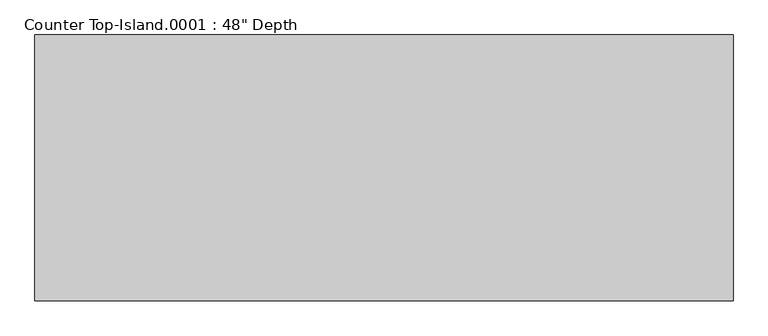
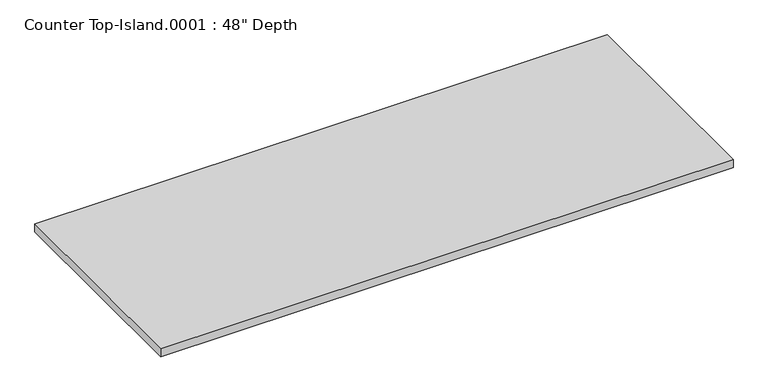
"""IFC4 building model written with IfcOpenShell, lengths in millimetres: furniture geometry."""

from ifc_helpers import new_model, si_unit, frame, origin, place, context, project, spatial, polyline, outline, extrude, source, transform, mapped, element, save


def furniture_be580aea(model_context):
    return source(origin(), model_context, "Body", "SweptSolid", [
        extrude(outline(polyline([(1403.0377049, 25.4), (1403.0377049, -965.4575383), (-1200.4622951, -965.4575383), (-1200.4622951, 25.4), (1403.0377049, 25.4)])), frame((0.0, 0.0, 571.5), z_axis=(0.0, 0.0, 1.0), x_axis=(1.0, 0.0, 0.0)), (0.0, 0.0, 1.0), 38.1),
    ])


if __name__ == "__main__":
    model = new_model("IFC4")
    model_context = context("Model", 3, world=origin())
    ifc_project = project(units=[si_unit("LENGTHUNIT", "METRE", prefix="MILLI")], contexts=[model_context])
    site = spatial("IfcSite", under=ifc_project)
    building = spatial("IfcBuilding", under=site)
    placement = place(None, origin())
    furniture_shape = furniture_be580aea(model_context)
    element("IfcFurniture", 1, ObjectType="Counter Top-Island.0001 : 48\" Depth", at=placement, inside=building, context=model_context, shape_type="MappedRepresentation", body=[
        mapped(furniture_shape, transform((0.0, 0.0, 0.0), x_axis=(1.0, 0.0, 0.0), y_axis=(0.0, 1.0, 0.0), z_axis=(0.0, 0.0, 1.0))),
    ])
    save(model, "model.ifc")

# Revit data of these elements
# Type "Counter Top-Island.0001 : 48\" Depth"
#   Assembly Code = "C1030400"
#   Counter Thickness = 0' - 1 1/2"
#   Depth [instance default] = 4' - 2"
#   Height = 2' - 0"
#   Length [instance default] = 8' - 0"
#   Counter Top Material = none
#   Default Elevation = 0
# Element 1 (IfcFurniture, "Counter Top-Island.0001 : 48\" Depth")
#   Depth = 3' - 3.01014"
#   Length = 8' - 6 1/2"
#   Materials on its faces: "Counter Top"
# Materials
#   "Counter Top": class "Wood", colour RGB 226 177 128, transparency 0
